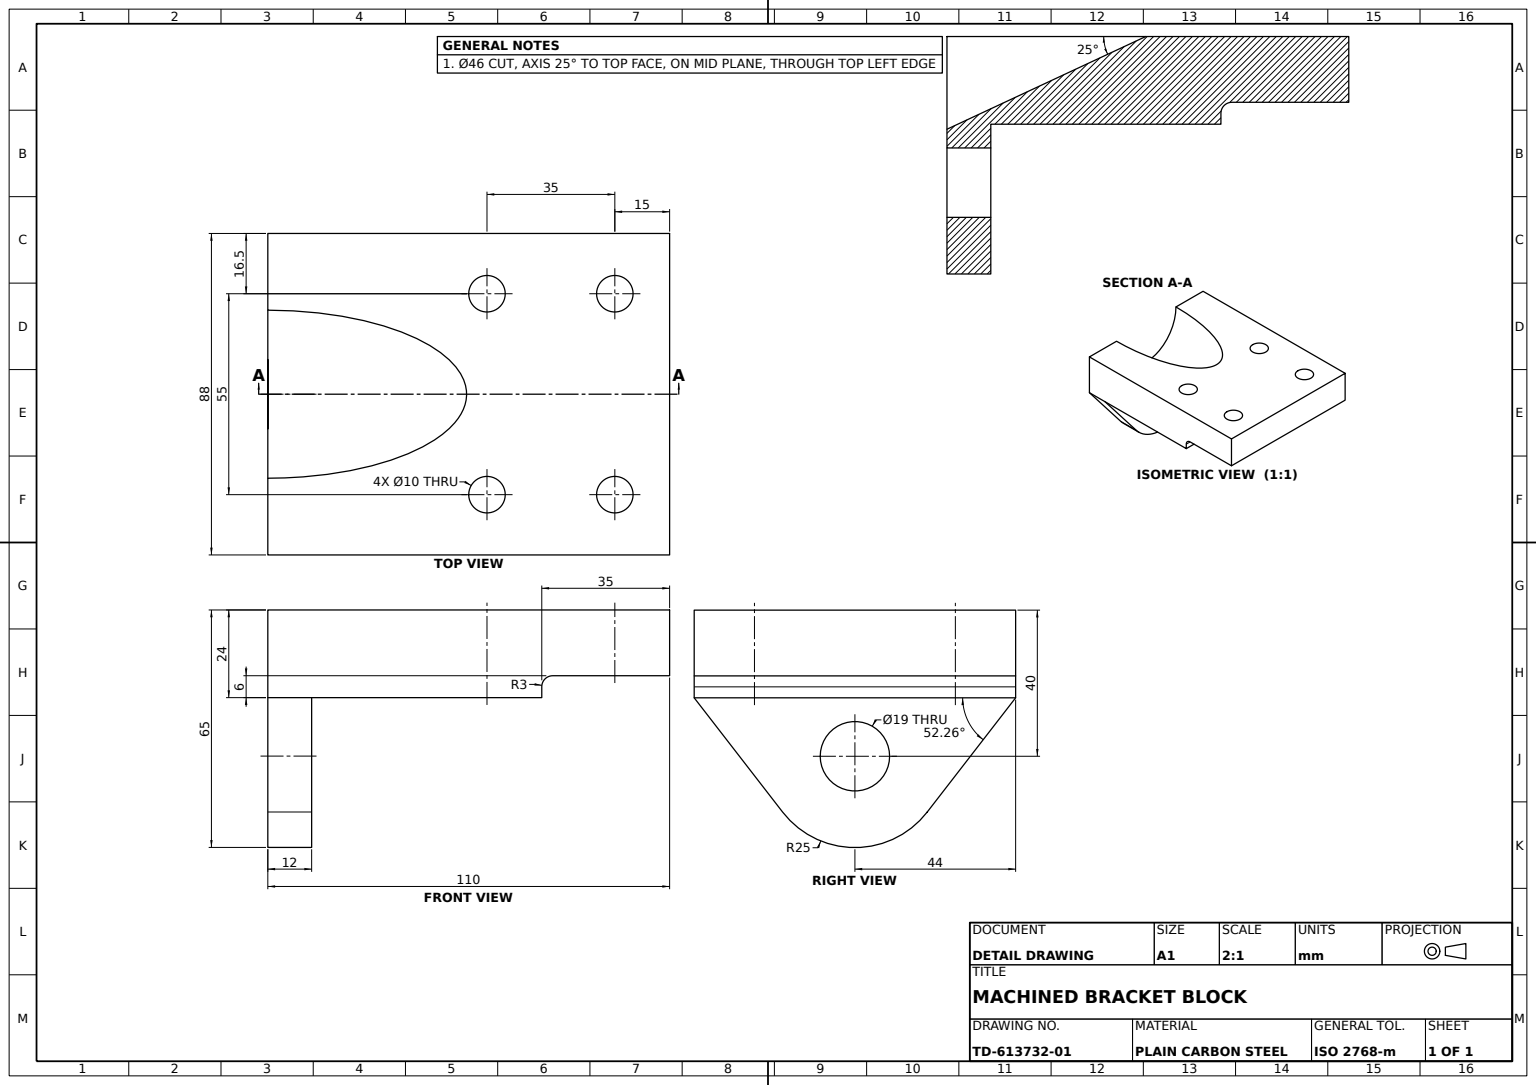
SolidWorks part; units mm, degrees
material "Plain Carbon Steel"
ref_plane "Front Plane" through (0, 0, 0) normal (0, 0, 1) x (1, 0, 0)
ref_plane "Top Plane" through (0, 0, 0) normal (0, 1, 0) x (1, 0, 0)
ref_plane "Right Plane" through (0, 0, 0) normal (1, 0, 0) x (0, 0, -1)
sketch "Body Profile Sketch" plane through (0, 0, 0) normal (0, 0, 1) x (1, 0, 0)
  line L0 (-44, 0) -> (44, 0)
  line L1 (44, 0) -> (44, -24)
  line L2 (44, -24) -> (19.7692, -55.3029)
  line L3 (-44, 0) -> (-44, -24)
  line L4 (-44, -24) -> (-19.7692, -55.3029)
  circle A0 centre (0, -40) radius 9.5
  circle A1 centre (0, -40) radius 25
  dimension "D3" = 19
  dimension "D4" = 50
  dimension "D1" = 88
  dimension "D2" = 44
  dimension "D5" = 24
  dimension "D6" = 24
  dimension "D7" = 40
  dimension "D8" = 0
extrude "Bracket Body Extrude 110" add sketch "Body Profile Sketch" against normal blind 110 contours A1 L2 L1 L0 L3 L4 | A1 A0
sketch "Through Slot Sketch" plane through (44, 0, 0) normal (1, 0, 0) x (0, 0, -1)
  line L0 (12, -76.36) -> (12, -24)
  line L1 (12, -24) -> (75, -24)
  line L2 (75, -24) -> (75, -21)
  line L3 (78, -18) -> (121.7714, -18)
  line L4 (0, -24) -> (0, -55.3029) construction
  line L5 (110, 0) -> (110, -24) construction
  line L6 (110, 0) -> (0, 0) construction
  line L7 (12, -76.36) -> (130.178, -76.36)
  line L8 (130.178, -76.36) -> (121.7714, -18)
  line L9 (0, 0) -> (0, -24) construction
  line L10 (110, -24) -> (0, -24) construction
  arc A0 (75, -21) -> (78, -18) centre (78, -21) cw
  dimension "D5" = 3
  dimension "D1" = 12
  dimension "D2" = 35
  dimension "D3" = 24
  dimension "D4" = 6
  dimension "D6" = 121.7714
  dimension "D7" = 130.178
  dimension "D8" = 52.36
extrude "Through Slot Cut" cut sketch "Through Slot Sketch" against normal blind 110
sketch "Bore Plane Reference Line 25deg" plane through (44, 0, 0) normal (1, 0, 0) x (0, 0, -1)
  line L0 (0, -25.3777) -> (104.3514, 23.2822)
  line L1 (0, 0) -> (0, -24) construction
  line L2 (110, 0) -> (0, 0) construction
  line L3 (75, -21) -> (75, -24) construction
  dimension "D1" = 25
  dimension "D2" = 23
  dimension "D3" = 29.3514
ref_plane "Angled Bore Plane" through (0, 0, 0) normal (0, 0.4226, -0.9063) x (-1, 0, 0)
sketch "Angled Bore Sketch Ø46" plane through (0, 0, 0) normal (0, 0.4226, -0.9063) x (-1, 0, 0)
  circle A0 centre (0, 0) radius 23
  dimension "D1" = 46
extrude "Angled Bore Ø46" cut sketch "Angled Bore Sketch Ø46" against normal mid plane 110
sketch "Mounting Holes Sketch" plane through (0, 0, 0) normal (0, 1, 0) x (1, 0, 0)
  line L0 (-44, 110) -> (44, 110) construction
  circle A0 centre (-27.5, 95) radius 5
  circle A1 centre (-27.5, 60) radius 5
  circle A2 centre (27.5, 60) radius 5
  circle A3 centre (27.5, 95) radius 5
  dimension "D1" = 10
  dimension "D2" = 10
  dimension "D3" = 10
  dimension "D4" = 10
  dimension "D5" = 35
  dimension "D6" = 35
  dimension "D7" = 55
  dimension "D8" = 27.5
  dimension "D9" = 15
  dimension "D10" = 15
extrude "Mounting Holes 4xØ10" cut sketch "Mounting Holes Sketch" against normal mid plane 110
